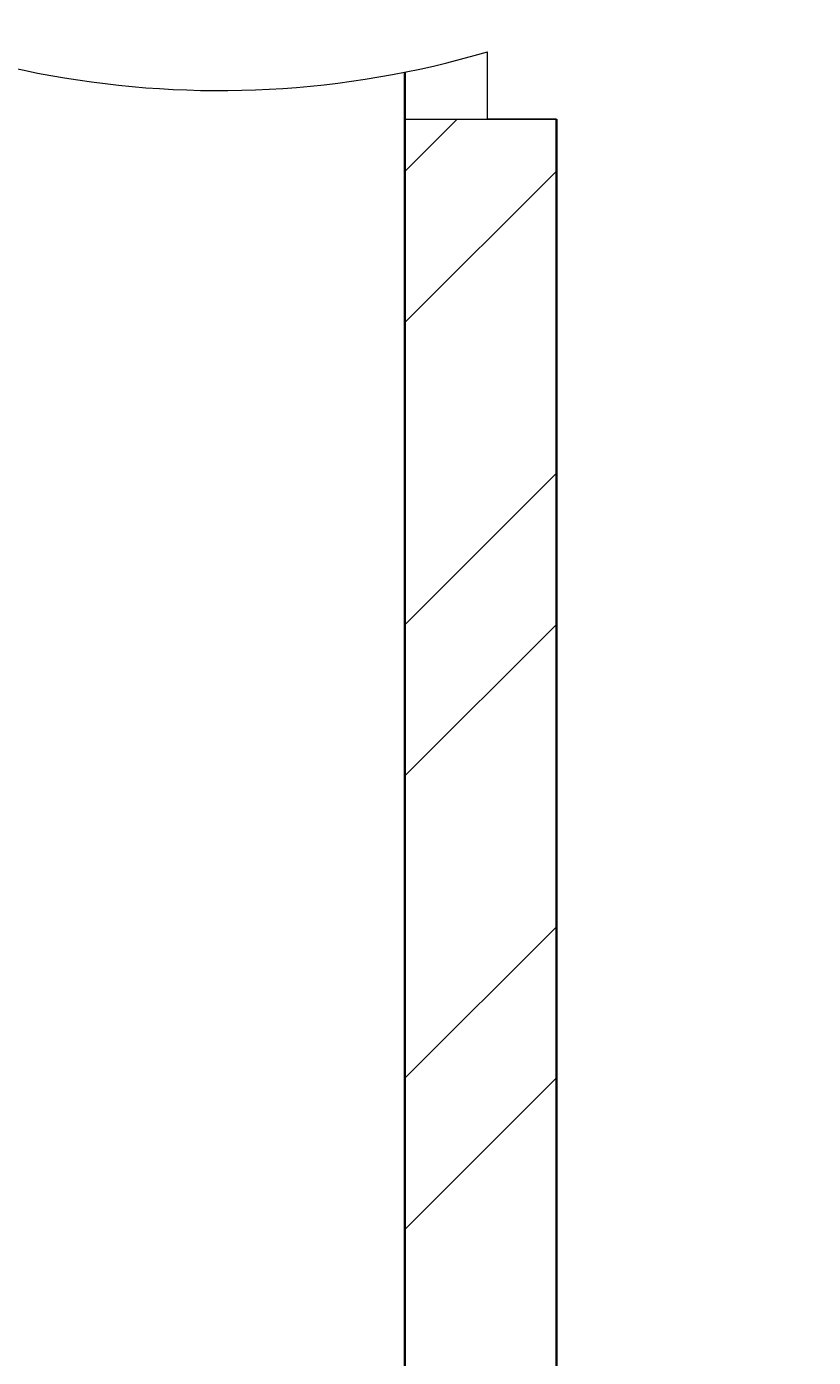
# Model space of a CAD drawing. Units: inches. Extents: x 1962 to 2771, y 1245 to 2660.
# Tile 57 of 114: x 2224 to 2247, y 2105 to 2145. Entities that reach past the tile are written whole.
import ezdxf

# ---------------------------------------------------------------- set-up
doc = ezdxf.new("R2010")
doc.units = ezdxf.units.IN
for name, color, linetype, lineweight in [('A-ANNO-DIMS', 2, 'Continuous', 18), ('A-DOOR', 3, 'Continuous', 18), ('A-WALL', 7, 'Continuous', 35), ('A-WALL-PATT', 252, 'Continuous', 13)]:
    doc.layers.add(name, color=color, linetype=linetype, lineweight=lineweight)
doc.styles.get("Standard").update_dxf_attribs({"font": 'arial.ttf'})
doc.dimstyles.get("Standard").update_dxf_attribs({"dimtxt": 0.18, "dimasz": 0.18, "dimexe": 0.18, "dimexo": 0.0625, "dimgap": 0.09, "dimtad": 0, "dimtih": 1, "dimtoh": 1, "dimdec": 4, "dimzin": 0, "dimdsep": 46, "dimtxsty": 'Standard', "dimcen": 0.09, "dimadec": 0, "dimazin": 0, "dimtfac": 1, "dimtdec": 4, "dimtofl": 0, "dimtmove": 0, "dimatfit": 3, "dimfxl": 1, "dimtolj": 1, "dimtzin": 0, "dimarcsym": 0})

# ---------------------------------------------------------------- blocks, each defined once
blk = doc.blocks.new('*D40')
at = {"layer": 'A-ANNO-DIMS', "color": 0, "lineweight": -2, "transparency": 16777216}
for p, q in [((2072.02, 2033.906), (2072.02, 2583.474)), ((2072.2, 2583.294), (2366.02, 2583.294)), ((2660.627, 2583.294), (2366.808, 2583.294)), ((2660.807, 2524.406), (2660.807, 2583.474))]:
    blk.add_line(p, q, dxfattribs=at)
at = {"layer": 'A-ANNO-DIMS', "color": 0, "transparency": 16777216}
for points in [[(2072.2, 2583.324), (2072.2, 2583.264), (2072.02, 2583.294)], [(2660.627, 2583.324), (2660.627, 2583.264), (2660.807, 2583.294)]]:
    blk.add_solid(points, dxfattribs=at)
at = {"layer": 'Defpoints', "color": 0, "transparency": 16777216}
for p in [(2660.807, 2583.294), (2660.807, 2524.344), (2072.02, 2033.844)]:
    blk.add_point(p, dxfattribs=at)
at = {"layer": 'A-ANNO-DIMS', "color": 0, "transparency": 16777216, "insert": (2366.414, 2583.294), "char_height": 0.18, "attachment_point": 5}
blk.add_mtext('\\A1;588.8', dxfattribs=at)

msp = doc.modelspace()

# ---------------------------------------------------------------- hatches: boundary and pattern name
at = {"layer": 'A-WALL-PATT'}
h = msp.add_hatch(dxfattribs=at)
h.set_pattern_fill('ANSI32', color=256)
h.paths.add_polyline_path([(2090.8074, 2467.3437), (2141.6481, 2467.3437), (2141.6481, 2469.5937), (2141.6481, 2471.8437), (2086.3074, 2471.8437), (2086.3074, 2422.5333), (2090.8074, 2422.5333)])
h.paths.add_polyline_path([(2282.7664, 2471.8437), (2204.8982, 2471.8437), (2204.8982, 2467.3437), (2234.8074, 2467.3437), (2234.8074, 2311.3437), (2228.7492, 2311.3437), (2228.7492, 2306.8437), (2234.8074, 2306.8437), (2331.9227, 2306.8437), (2331.9227, 2309.0937), (2331.9227, 2311.3437), (2239.3074, 2311.3437), (2239.3074, 2467.3437), (2282.7664, 2467.3437), (2282.7664, 2469.5937)])
h.paths.add_polyline_path([(2471.4531, 2519.8437), (2552.011, 2519.8437), (2564.3996, 2519.8437), (2564.3996, 2511.1389), (2568.8996, 2511.1389), (2568.8996, 2524.3437), (2466.9531, 2524.3437), (2466.9531, 2471.8437), (2450.0749, 2471.8437), (2446.4672, 2471.8437), (2446.4672, 2467.3437), (2450.0749, 2467.3437), (2475.9988, 2467.3437), (2475.9988, 2469.5937), (2475.9988, 2471.8437), (2471.4531, 2471.8437)])
h.paths.add_polyline_path([(2575.2231, 2469.5937), (2575.2231, 2471.8437), (2568.8996, 2471.8437), (2568.8996, 2487.1389), (2564.3996, 2487.1389), (2564.3996, 2471.8437), (2556.511, 2471.8437), (2499.2904, 2471.8437), (2499.2904, 2467.3437), (2507.8074, 2467.3437), (2507.8074, 2311.3437), (2414.863, 2311.3437), (2414.863, 2306.8437), (2512.3074, 2306.8437), (2517.0114, 2306.8437), (2517.0114, 2309.0937), (2517.0114, 2311.3437), (2512.3074, 2311.3437), (2512.3074, 2467.3437), (2575.2231, 2467.3437)])
h.paths.add_polyline_path([(2660.8074, 2471.8437), (2600.9602, 2471.8437), (2600.9602, 2467.3437), (2656.3074, 2467.3437), (2656.3074, 2432.5704), (2660.8074, 2432.5704)])
h.paths.add_polyline_path([(2660.8074, 2372.5704), (2656.3074, 2372.5704), (2656.3074, 2311.3437), (2600.276, 2311.3437), (2600.276, 2309.0937), (2600.276, 2306.8437), (2656.3074, 2306.8437), (2656.3074, 2296.2593), (2660.8074, 2296.2593)])
h.paths.add_polyline_path([(2572.3074, 2306.8437), (2577.1385, 2306.8437), (2577.1385, 2311.3437), (2551.082, 2311.3437), (2551.082, 2306.8437), (2567.8074, 2306.8437), (2567.8074, 2258.8437), (2540.0574, 2258.8437), (2540.0574, 2256.5937), (2540.0574, 2254.3437), (2567.8074, 2254.3437), (2656.3074, 2254.3437), (2656.3074, 2236.9085), (2660.8074, 2236.9085), (2660.8074, 2272.2593), (2656.3074, 2272.2593), (2656.3074, 2258.8437), (2572.3074, 2258.8437)])
h.paths.add_polyline_path([(2512.3074, 2254.3437), (2518.8716, 2254.3437), (2518.8716, 2256.5937), (2518.8716, 2258.8437), (2507.8074, 2258.8437), (2507.8074, 2177.8437), (2567.8074, 2177.8437), (2567.8074, 2172.9628), (2572.3074, 2172.9628), (2572.3074, 2177.8437), (2656.3074, 2177.8437), (2656.3074, 2166.4846), (2660.8074, 2166.4846), (2660.8074, 2200.9085), (2656.3074, 2200.9085), (2656.3074, 2182.3437), (2512.3074, 2182.3437)])
h.paths.add_polyline_path([(2656.3074, 2129.8437), (2572.3074, 2129.8437), (2572.3074, 2150.3044), (2570.0574, 2150.3044), (2567.8074, 2150.3044), (2567.8074, 2129.8437), (2507.8074, 2129.8437), (2507.8074, 2116.3027), (2510.0574, 2116.3027), (2512.3074, 2116.3027), (2512.3074, 2125.3437), (2567.8074, 2125.3437), (2572.3074, 2125.3437), (2656.3074, 2125.3437)])
h.paths.add_polyline_path([(2090.8074, 2362.5333), (2086.3074, 2362.5333), (2086.3074, 2298.6242), (2090.8074, 2298.6242), (2090.8074, 2306.8437), (2174.8074, 2306.8437), (2174.8074, 2286.4178), (2179.3074, 2286.4178), (2179.3074, 2306.8437), (2192.8641, 2306.8437), (2192.8641, 2309.0937), (2192.8641, 2311.3437), (2090.8074, 2311.3437)])
h.paths.add_polyline_path([(2209.156, 2258.8437), (2179.3074, 2258.8437), (2179.3074, 2263.2236), (2177.0574, 2263.2236), (2174.8074, 2263.2236), (2174.8074, 2258.8437), (2090.8074, 2258.8437), (2090.8074, 2274.6242), (2086.3074, 2274.6242), (2086.3074, 2238.2967), (2088.5574, 2238.2967), (2090.8074, 2238.2967), (2090.8074, 2254.3437), (2209.156, 2254.3437)])
h.paths.add_polyline_path([(2090.8074, 2177.8437), (2234.8074, 2177.8437), (2234.8074, 2173.1428), (2239.3074, 2173.1428), (2239.3074, 2258.8437), (2230.8442, 2258.8437), (2230.8442, 2256.5937), (2230.8442, 2254.3437), (2234.8074, 2254.3437), (2234.8074, 2182.3437), (2090.8074, 2182.3437), (2090.8074, 2202.2967), (2086.3074, 2202.2967), (2086.3074, 2140.0389), (2090.8074, 2140.0389)])
h.paths.add_polyline_path([(2090.8074, 2080.0389), (2086.3074, 2080.0389), (2086.3074, 2033.8437), (2090.8074, 2033.8437)], flags=17)
h.paths.add_polyline_path([(2244.9405, 2033.8437), (2239.3074, 2033.8437), (2239.3074, 2142.0665), (2237.2592, 2142.0665), (2234.8074, 2142.0665), (2234.8074, 2033.8437), (2090.8074, 2033.8437), (2076.5204, 2033.8437), (2072.0204, 2033.8437), (2072.0204, 2000.4493), (2076.5204, 2000.4493), (2076.5204, 2029.3437), (2090.8074, 2029.3437), (2244.9405, 2029.3437), (2244.9405, 2031.5937)])
h.paths.add_polyline_path([(2234.8074, 1933.3437), (2076.5204, 1933.3437), (2076.5204, 1952.4493), (2074.2704, 1952.4493), (2072.0204, 1952.4493), (2072.0204, 1933.3437), (2072.0204, 1928.8437), (2234.8074, 1928.8437)])
h.paths.add_polyline_path([(2090.8074, 1928.8437), (2086.3074, 1928.8437), (2086.3074, 1906.5013), (2090.8074, 1906.5013)])
h.paths.add_polyline_path([(2090.8074, 1846.5013), (2086.3074, 1846.5013), (2086.3074, 1769.9917), (2088.5574, 1769.9917), (2090.8074, 1769.9917), (2090.8074, 1780.3437), (2234.8074, 1780.3437), (2234.8074, 1708.3437), (2230.3764, 1708.3437), (2230.3764, 1703.8437), (2239.3074, 1703.8437), (2239.3074, 1792.6669), (2237.0574, 1792.6669), (2234.8074, 1792.6669), (2234.8074, 1784.8437), (2090.8074, 1784.8437)])
h.paths.add_polyline_path([(2239.3074, 1928.8437), (2244.9405, 1928.8437), (2244.9405, 1931.0937), (2244.9405, 1933.3437), (2234.8074, 1933.3437), (2234.8074, 1928.8437), (2234.8074, 1825.5949), (2239.3074, 1825.5949)])
h.paths.add_polyline_path([(2148.0425, 1649.0937), (2148.0425, 1651.3437), (2090.8074, 1651.3437), (2090.8074, 1646.8437), (2148.0425, 1646.8437)], flags=0)
h.paths.add_polyline_path([(2207.5601, 1708.3437), (2090.8074, 1708.3437), (2090.8074, 1703.8437), (2174.8074, 1703.8437), (2174.8074, 1651.3437), (2170.4457, 1651.3437), (2170.4457, 1646.8437), (2195.9924, 1646.8437), (2195.9924, 1649.0937), (2195.9924, 1651.3437), (2179.3074, 1651.3437), (2179.3074, 1703.8437), (2207.5601, 1703.8437), (2207.5601, 1706.0937)])
h.paths.add_polyline_path([(2090.8074, 1733.9917), (2086.3074, 1733.9917), (2086.3074, 1696.1032), (2088.5574, 1696.1032), (2090.8074, 1696.1032)])
h.paths.add_polyline_path([(2090.8074, 1672.1032), (2086.3074, 1672.1032), (2086.3074, 1600.3335), (2090.8074, 1600.3335)])
h.paths.add_polyline_path([(2090.8074, 1540.3335), (2086.3074, 1540.3335), (2086.3074, 1486.3437), (2139.6766, 1486.3437), (2139.6766, 1490.8437), (2090.8074, 1490.8437)])
h.paths.add_polyline_path([(2302.3876, 1490.8437), (2239.3074, 1490.8437), (2239.3074, 1646.8437), (2335.9994, 1646.8437), (2335.9994, 1651.3437), (2229.884, 1651.3437), (2229.884, 1646.8437), (2234.8074, 1646.8437), (2234.8074, 1490.8437), (2202.7103, 1490.8437), (2202.7103, 1488.5937), (2202.7103, 1486.3437), (2275.0699, 1486.3437), (2275.0699, 1475.772), (2279.5699, 1475.772), (2279.5699, 1486.3437), (2302.3876, 1486.3437)])
h.paths.add_polyline_path([(2279.5699, 1451.772), (2275.0699, 1451.772), (2275.0699, 1438.3437), (2174.8074, 1438.3437), (2174.8074, 1486.3437), (2179.7922, 1486.3437), (2179.7922, 1490.8437), (2163.3585, 1490.8437), (2163.3585, 1488.5937), (2163.3585, 1486.3437), (2170.3074, 1486.3437), (2170.3074, 1433.8437), (2279.5699, 1433.8437)])
h.paths.add_polyline_path([(2427.2363, 1490.8437), (2375.8074, 1490.8437), (2375.8074, 1646.8437), (2381.6401, 1646.8437), (2381.6401, 1651.3437), (2365.887, 1651.3437), (2365.887, 1649.0937), (2365.887, 1646.8437), (2371.3074, 1646.8437), (2371.3074, 1490.8437), (2327.5627, 1490.8437), (2327.5627, 1488.5937), (2327.5627, 1486.3437), (2371.3074, 1486.3437), (2371.3074, 1433.8437), (2375.8074, 1433.8437), (2375.8074, 1486.3437), (2427.2363, 1486.3437)])
h.paths.add_polyline_path([(2512.3074, 1646.8437), (2519.4351, 1646.8437), (2519.4351, 1649.0937), (2519.4351, 1651.3437), (2507.8074, 1651.3437), (2416.0063, 1651.3437), (2416.0063, 1649.0937), (2416.0063, 1646.8437), (2507.8074, 1646.8437), (2507.8074, 1490.8437), (2497.0532, 1490.8437), (2497.0532, 1488.5937), (2497.0532, 1486.3437), (2574.9344, 1486.3437), (2574.9344, 1476.0181), (2579.4344, 1476.0181), (2579.4344, 1486.3437), (2584.4872, 1486.3437), (2584.3074, 1490.8437), (2512.3074, 1490.8437)])
h.paths.add_polyline_path([(2470.5091, 1486.3437), (2473.9767, 1486.3437), (2473.9767, 1490.8437), (2449.6605, 1490.8437), (2449.6605, 1488.5937), (2449.6605, 1486.3437), (2466.0091, 1486.3437), (2466.0091, 1433.8437), (2470.5091, 1433.8437), (2579.4344, 1433.8437), (2579.4344, 1452.0181), (2574.9344, 1452.0181), (2574.9344, 1438.3437), (2554.5091, 1438.3437), (2470.5091, 1438.3437)])
h.paths.add_polyline_path([(2656.3074, 1490.8437), (2611.86, 1490.8437), (2611.86, 1486.3437), (2656.3074, 1486.3437)])
h.paths.add_polyline_path([(2660.8074, 1532.7007), (2658.5574, 1532.7007), (2656.3074, 1532.7007), (2656.3074, 1486.3437), (2660.8074, 1486.3437)])
h.paths.add_polyline_path([(2660.8074, 1664.9663), (2656.3074, 1664.9663), (2656.3074, 1651.3437), (2602.2313, 1651.3437), (2602.2313, 1646.8437), (2656.3074, 1646.8437), (2656.3074, 1592.7007), (2660.8074, 1592.7007)])
h.paths.add_polyline_path([(2660.8074, 1724.5221), (2656.3074, 1724.5221), (2656.3074, 1703.8437), (2542.4725, 1703.8437), (2542.4725, 1699.3437), (2567.8074, 1699.3437), (2567.8074, 1651.3437), (2552.7766, 1651.3437), (2552.7766, 1649.0937), (2552.7766, 1646.8437), (2577.2878, 1646.8437), (2577.2878, 1649.0937), (2577.2878, 1651.3437), (2572.3074, 1651.3437), (2572.3074, 1699.3437), (2656.3074, 1699.3437), (2656.3074, 1688.9663), (2660.8074, 1688.9663)])
h.paths.add_polyline_path([(2660.8074, 1880.6524), (2656.3074, 1880.6524), (2656.3074, 1832.8437), (2512.3074, 1832.8437), (2512.3074, 1837.8959), (2507.8074, 1837.8959), (2507.8074, 1828.3437), (2567.8074, 1828.3437), (2567.8074, 1804.3437), (2572.3074, 1804.3437), (2572.3074, 1828.3437), (2656.3074, 1828.3437), (2656.3074, 1818.6778), (2660.8074, 1818.6778)])
h.paths.add_polyline_path([(2660.8074, 1794.6778), (2656.3074, 1794.6778), (2656.3074, 1780.3437), (2572.3074, 1780.3437), (2572.3074, 1783.0303), (2570.0574, 1783.0303), (2567.8074, 1783.0303), (2567.8074, 1780.3437), (2507.8074, 1780.3437), (2507.8074, 1699.3437), (2517.8858, 1699.3437), (2517.8858, 1701.5937), (2517.8858, 1703.8437), (2512.3074, 1703.8437), (2512.3074, 1775.8437), (2656.3074, 1775.8437), (2656.3074, 1760.5221), (2660.8074, 1760.5221)])
h.paths.add_polyline_path([(2660.8074, 1981.3437), (2660.8074, 2020.2808), (2658.5574, 2020.2808), (2656.3074, 2020.2808), (2656.3074, 1981.3437), (2512.3074, 1981.3437), (2512.3074, 2086.6996), (2507.8074, 2086.6996), (2507.8074, 1981.3437), (2375.8074, 1981.3437), (2375.8074, 1986.8505), (2373.5574, 1986.8505), (2371.3074, 1986.8505), (2371.3074, 1973.2607), (2375.8074, 1973.2607), (2375.8074, 1976.8437), (2507.8074, 1976.8437), (2507.8074, 1865.4281), (2510.0574, 1865.4281), (2512.3074, 1865.4281), (2512.3074, 1976.8437), (2660.8074, 1976.8437)])
h.paths.add_polyline_path([(2375.8074, 1940.297), (2373.5574, 1940.297), (2371.3074, 1940.297), (2371.3074, 1933.3437), (2278.4434, 1933.3437), (2278.4434, 1928.8437), (2371.3074, 1928.8437), (2371.3074, 1651.3437), (2375.8074, 1651.3437)])
h.paths.add_polyline_path([(2660.8074, 1976.8437), (2656.3074, 1976.8437), (2656.3074, 1940.6524), (2660.8074, 1940.6524)], flags=17)
h.paths.add_polyline_path([(2660.8074, 2142.4846), (2656.3074, 2142.4846), (2656.3074, 2080.2808), (2660.8074, 2080.2808)])
h.paths.add_polyline_path([(2381.4189, 2311.3437), (2375.8074, 2311.3437), (2375.8074, 2467.3437), (2424.7242, 2467.3437), (2424.7242, 2469.5937), (2424.7242, 2471.8437), (2375.8074, 2471.8437), (2375.8074, 2524.3437), (2371.3074, 2524.3437), (2371.3074, 2471.8437), (2307.2097, 2471.8437), (2307.2097, 2467.3437), (2371.3074, 2467.3437), (2371.3074, 2311.3437), (2366.8901, 2311.3437), (2366.8901, 2306.8437), (2371.3074, 2306.8437), (2371.3074, 2033.8437), (2279.6589, 2033.8437), (2279.6589, 2029.3437), (2371.3074, 2029.3437), (2371.3074, 2014.2598), (2375.8074, 2014.2598), (2375.8074, 2306.8437), (2381.4189, 2306.8437)])
h.paths.add_polyline_path([(2263.3074, 2524.3437), (2170.3074, 2524.3437), (2170.3074, 2519.8437), (2170.3074, 2471.8437), (2165.0312, 2471.8437), (2165.0312, 2467.3437), (2179.6721, 2467.3437), (2179.6721, 2469.5161), (2179.6721, 2471.8437), (2174.8074, 2471.8437), (2174.8074, 2519.8437), (2258.8074, 2519.8437), (2258.8074, 2511.6436), (2263.3074, 2511.6436)])
h.paths.add_polyline_path([(2245.0232, 1361.4123), (2492.9468, 1361.4123), (2492.9468, 1398.505), (2245.0232, 1398.505)], flags=9)
h.paths.add_polyline_path([(2388.1434, 2086.6936), (2425.0704, 2086.6936), (2425.0704, 2105.3509), (2388.1434, 2105.3509)], flags=9)
h.paths.add_polyline_path([(2404.922, 2242.6744), (2445.7337, 2242.6744), (2445.7337, 2261.3318), (2404.922, 2261.3318)], flags=9)
h.paths.add_polyline_path([(2269.4107, 2156.7935), (2306.3378, 2156.7935), (2306.3378, 2175.4508), (2269.4107, 2175.4508)], flags=9)
h.paths.add_polyline_path([(2269.3277, 2233.4343), (2306.2547, 2233.4343), (2306.2547, 2252.0917), (2269.3277, 2252.0917)], flags=9)
h.paths.add_polyline_path([(2431.6052, 2320.6922), (2470.4456, 2320.6922), (2470.4456, 2339.3495), (2431.6052, 2339.3495)], flags=25)
h.paths.add_polyline_path([(2249.6902, 2315.7608), (2288.5306, 2315.7608), (2288.5306, 2334.4182), (2249.6902, 2334.4182)], flags=25)
h.paths.add_polyline_path([(2096.9301, 2314.3181), (2135.7704, 2314.3181), (2135.7704, 2332.9755), (2096.9301, 2332.9755)], flags=25)
h.paths.add_polyline_path([(2134.3475, 2285.7089), (2161.4655, 2285.7089), (2161.4655, 2304.3662), (2134.3475, 2304.3662)], flags=9)
h.paths.add_polyline_path([(2126.5155, 2209.4076), (2159.9227, 2209.4076), (2159.9227, 2228.065), (2126.5155, 2228.065)], flags=25)
h.paths.add_polyline_path([(2110.5753, 2141.5299), (2149.4157, 2141.5299), (2149.4157, 2160.1872), (2110.5753, 2160.1872)], flags=25)
h.paths.add_polyline_path([(2249.8618, 1968.3317), (2286.3966, 1968.3317), (2286.3966, 1986.989), (2249.8618, 1986.989)], flags=9)
h.paths.add_polyline_path([(2395.9507, 1777.0051), (2436.7624, 1777.0051), (2436.7624, 1795.6625), (2395.9507, 1795.6625)], flags=9)
h.paths.add_polyline_path([(2398.5259, 1888.5651), (2435.0062, 1888.5651), (2435.0062, 1907.2224), (2398.5259, 1907.2224)], flags=25)
h.paths.add_polyline_path([(2259.3506, 1728.3559), (2296.2776, 1728.3559), (2296.2776, 1747.0132), (2259.3506, 1747.0132)], flags=9)
h.paths.add_polyline_path([(2271.3698, 1845.268), (2308.2968, 1845.268), (2308.2968, 1863.9253), (2271.3698, 1863.9253)], flags=9)
h.paths.add_polyline_path([(2120.9355, 1786.3027), (2159.7759, 1786.3027), (2159.7759, 1804.9601), (2120.9355, 1804.9601)], flags=25)
h.paths.add_polyline_path([(2121.3164, 1732.1043), (2154.7236, 1732.1043), (2154.7236, 1750.7616), (2121.3164, 1750.7616)], flags=25)
h.paths.add_polyline_path([(2118.3706, 1678.8997), (2147.5282, 1678.8997), (2147.5282, 1697.557), (2118.3706, 1697.557)], flags=25)
h.paths.add_polyline_path([(2385.9227, 1493.557), (2424.763, 1493.557), (2424.763, 1512.2143), (2385.9227, 1512.2143)], flags=25)
h.paths.add_polyline_path([(2248.7058, 1500.0256), (2287.5462, 1500.0256), (2287.5462, 1518.6829), (2248.7058, 1518.6829)], flags=25)
h.paths.add_polyline_path([(2104.1669, 1617.3771), (2143.0073, 1617.3771), (2143.0073, 1636.0344), (2104.1669, 1636.0344)], flags=9)
h.paths.add_polyline_path([(2096.0714, 1447.8824), (2137.3845, 1447.8824), (2137.3845, 1458.1859), (2096.0714, 1458.1859)], flags=9)
h.paths.add_polyline_path([(2180.6114, 1440.325), (2209.7689, 1440.325), (2209.7689, 1458.9823), (2180.6114, 1458.9823)], flags=25)
h.paths.add_polyline_path([(2316.1698, 1447.9637), (2357.4829, 1447.9637), (2357.4829, 1458.2673), (2316.1698, 1458.2673)], flags=9)
h.paths.add_polyline_path([(2397.6187, 1447.9637), (2438.9318, 1447.9637), (2438.9318, 1458.2673), (2397.6187, 1458.2673)], flags=9)
h.paths.add_polyline_path([(2473.0778, 1439.5953), (2502.2354, 1439.5953), (2502.2354, 1458.2527), (2473.0778, 1458.2527)], flags=25)
h.paths.add_polyline_path([(2589.7027, 1447.8819), (2631.0158, 1447.8819), (2631.0158, 1458.1855), (2589.7027, 1458.1855)], flags=9)
h.paths.add_polyline_path([(2522.4009, 1497.5285), (2561.2413, 1497.5285), (2561.2413, 1516.1859), (2522.4009, 1516.1859)], flags=25)
h.paths.add_polyline_path([(2579.6565, 1671.3482), (2608.8141, 1671.3482), (2608.8141, 1690.0056), (2579.6565, 1690.0056)], flags=25)
h.paths.add_polyline_path([(2544.7038, 1725.5064), (2578.1111, 1725.5064), (2578.1111, 1744.1637), (2544.7038, 1744.1637)], flags=25)
h.paths.add_polyline_path([(2578.1191, 1807.472), (2607.2766, 1807.472), (2607.2766, 1826.1293), (2578.1191, 1826.1293)], flags=25)
h.paths.add_polyline_path([(2595.0614, 1835.1839), (2633.9018, 1835.1839), (2633.9018, 1853.8413), (2595.0614, 1853.8413)], flags=25)
h.paths.add_polyline_path([(2567.0097, 2097.7035), (2605.8501, 2097.7035), (2605.8501, 2116.3609), (2567.0097, 2116.3609)], flags=9)
h.paths.add_polyline_path([(2586.644, 2134.6454), (2615.8015, 2134.6454), (2615.8015, 2153.3027), (2586.644, 2153.3027)], flags=9)
h.paths.add_polyline_path([(2544.6185, 2212.6783), (2578.0258, 2212.6783), (2578.0258, 2231.3356), (2544.6185, 2231.3356)], flags=25)
h.paths.add_polyline_path([(2577.0273, 2256.9023), (2606.1849, 2256.9023), (2606.1849, 2275.5597), (2577.0273, 2275.5597)], flags=24)
h.paths.add_polyline_path([(2605.2683, 2315.2821), (2644.1087, 2315.2821), (2644.1087, 2333.9395), (2605.2683, 2333.9395)], flags=25)
h.paths.add_polyline_path([(2583.1244, 2496.1815), (2624.4375, 2496.1815), (2624.4375, 2506.4851), (2583.1244, 2506.4851)], flags=9)
h.paths.add_polyline_path([(2474.761, 2497.0823), (2503.9185, 2497.0823), (2503.9185, 2515.7397), (2474.761, 2515.7397)], flags=25)
h.paths.add_polyline_path([(2387.5787, 2494.2563), (2428.902, 2494.2563), (2428.902, 2504.5598), (2387.5787, 2504.5598)], flags=9)
h.paths.add_polyline_path([(2300.1657, 2500.1564), (2341.4788, 2500.1564), (2341.4788, 2510.46), (2300.1657, 2510.46)], flags=25)
h.paths.add_polyline_path([(2176.8589, 2497.5843), (2206.0165, 2497.5843), (2206.0165, 2516.2416), (2176.8589, 2516.2416)], flags=25)
h.paths.add_polyline_path([(2097.4668, 2494.9762), (2138.7799, 2494.9762), (2138.7799, 2505.2798), (2097.4668, 2505.2798)], flags=9)

# ---------------------------------------------------------------- linework, layer by layer
at = {"layer": 'A-DOOR'}
for p, q in [((2237.2592, 2142.0665), (2237.2592, 2144.0665)), ((2234.8074, 2142.0665), (2237.2592, 2142.0665)), ((2237.2592, 2142.0665), (2237.2592, 2142.0665)), ((2237.2592, 2142.0665), (2239.3074, 2142.0665)), ((2239.3074, 2142.0665), (2237.2592, 2142.0665))]:
    msp.add_line(p, q, dxfattribs=at)
msp.add_arc((2229.2838, 2171.1428), 28.2264, 180, 286.41252, dxfattribs=at)
at = {"layer": 'A-WALL'}
for p, q in [((2234.8074, 2143.4621), (2234.8074, 2033.8437)), ((2239.3074, 2142.0665), (2239.3074, 2033.8437))]:
    msp.add_line(p, q, dxfattribs=at)

# ---------------------------------------------------------------- dimensions: what is measured, and where the dimension line sits
at = {"layer": 'A-ANNO-DIMS'}
dim = msp.add_linear_dim(base=(2660.8074, 2583.2937), p1=(2072.0204, 2033.8437), p2=(2660.8074, 2524.3437), dimstyle='Standard', override={"dimdec": 1, "dimlfac": 1, "dimrnd": 0, "dimzin": 0, "dimdsep": 46, "dimlunit": 2}, dxfattribs=at)
dim.commit()
dim.dimension.update_dxf_attribs({"geometry": '*D40', "text_midpoint": (2366.4139, 2583.2937)})

doc.saveas('drawing.dxf')
